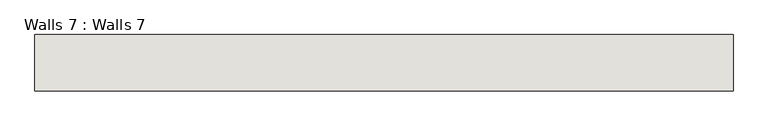
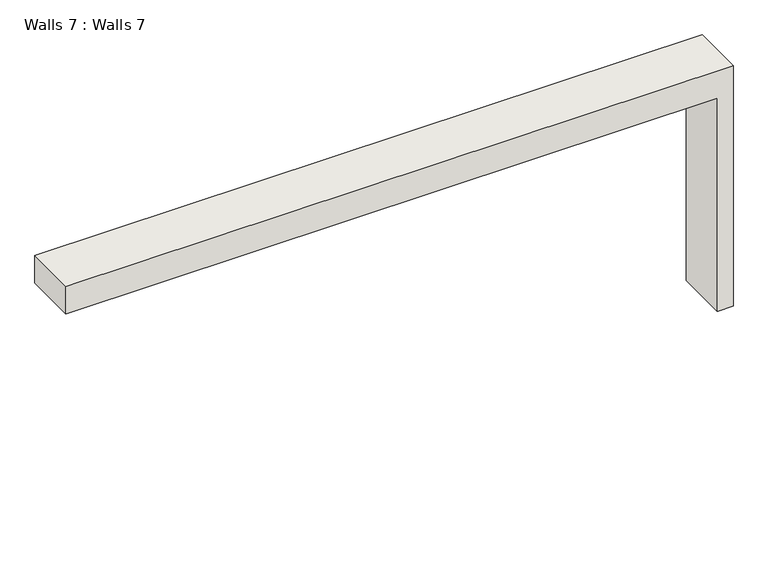
"""IFC4 building model written with IfcOpenShell, lengths in millimetres: wall geometry, Walls 7 : Walls 7."""

from ifc_helpers import new_model, si_unit, frame, origin, place, context, project, spatial, polyline, outline, extrude, source, transform, mapped, element, save


def walls_7_walls_7_71d3a732(model_context):
    return source(origin(), model_context, "Body", "SweptSolid", [
        extrude(outline(polyline([(3254.9841512, 1204.9616643), (3254.9841512, -7329.4383357), (2884.2980296, -7329.4383357), (2884.2980296, 1004.9616643), (0.0, 1004.9616643), (0.0, 1204.9616643), (3254.9841512, 1204.9616643)])), frame((0.0, -20618.075595, 0.0), z_axis=(0.0, 1.0, 0.0), x_axis=(0.0, 0.0, 1.0)), (0.0, 0.0, 1.0), 687.1545613),
    ])


if __name__ == "__main__":
    model = new_model("IFC4")
    model_context = context("Model", 3, world=origin())
    ifc_project = project(units=[si_unit("LENGTHUNIT", "METRE", prefix="MILLI")], contexts=[model_context])
    site = spatial("IfcSite", under=ifc_project)
    building = spatial("IfcBuilding", under=site)
    placement = place(None, origin())
    walls_7_walls_7_shape = walls_7_walls_7_71d3a732(model_context)
    element("IfcWall", 1, ObjectType="Walls 7 : Walls 7", at=placement, inside=building, context=model_context, shape_type="MappedRepresentation", body=[
        mapped(walls_7_walls_7_shape, transform((0.0, 0.0, 0.0), x_axis=(1.0, 0.0, 0.0), y_axis=(0.0, 1.0, 0.0), z_axis=(0.0, 0.0, 1.0))),
    ])
    save(model, "model.ifc")

# Revit data of these elements
# Element 1 (IfcWall, "Walls 7 : Walls 7")
#   Materials on its faces: "Default Wall"
# Materials
#   "Default Wall": colour RGB 80 80 80, transparency 0
